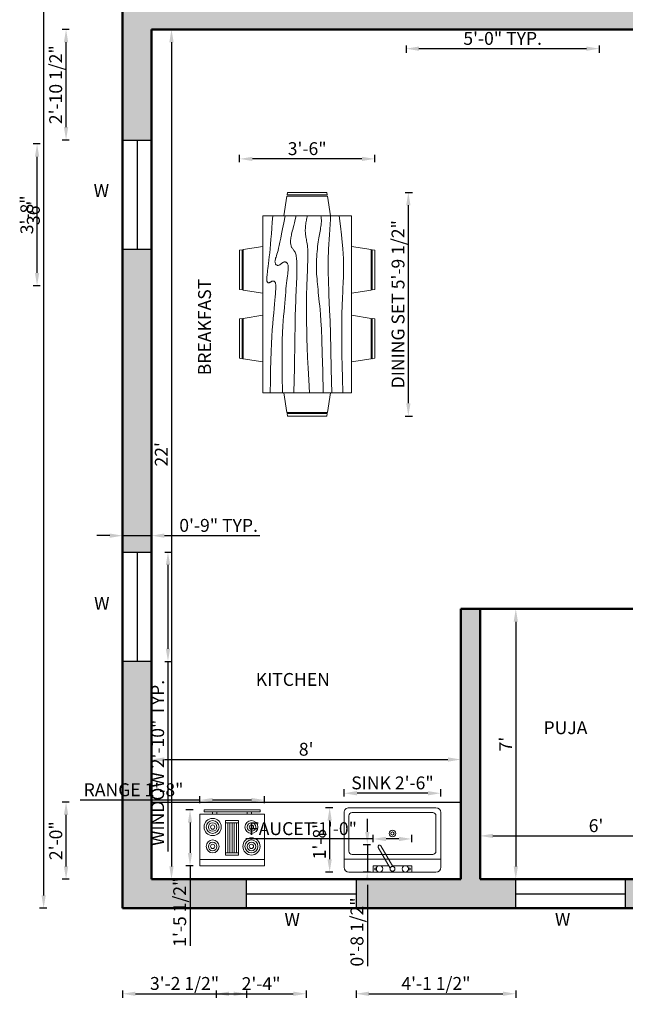
# Model space of a CAD drawing. Units: inches. Extents: x -31 to 511, y -453 to 49.
# Tile 1 of 4: x -31 to 157, y -448 to -142. Entities that reach past the tile are written whole.
import ezdxf

# ---------------------------------------------------------------- set-up
doc = ezdxf.new("R2010")
doc.units = ezdxf.units.IN
for name, color, linetype, lineweight in [('A-ANNO-DIMS', 2, 'Continuous', 18), ('A-ANNO-TEXT', 7, 'Continuous', 18), ('A-AREA-IDEN', 7, 'Continuous', 25), ('A-EQPM', 8, 'Continuous', 18), ('A-FLOR-CASE', 8, 'Continuous', 25), ('A-FLOR-FIXT', 9, 'Continuous', 18), ('A-FURN', 8, 'Continuous', 18), ('A-GLAZ', 4, 'Continuous', 25), ('A-WALL', 7, 'Continuous', 50), ('A-WALL-PATT', 252, 'Continuous', 13)]:
    doc.layers.add(name, color=color, linetype=linetype, lineweight=lineweight)
doc.styles.get("Standard").update_dxf_attribs({"font": 'arial.ttf'})
doc.dimstyles.new('ISO-25', dxfattribs={"dimtxt": 4, "dimasz": 4, "dimexe": 1.25, "dimexo": 0.625, "dimtad": 1, "dimlunit": 3, "dimtxsty": 'Standard', "dimcen": 2.5, "dimadec": 0, "dimazin": 0, "dimtfac": 1, "dimtmove": 0, "dimatfit": 3, "dimfxl": 1, "dimfxlon": 1, "dimarcsym": 0})

# ---------------------------------------------------------------- blocks, each defined once
blk = doc.blocks.new('Sink-single - 30 in top')
blk.add_line((-15, -3.999996), (15, -3.999996))
for points in [[(-13.5, 0), (13.5, 0)], [(-15, -18.499996), (-15, -1.5)], [(15, -1.5), (15, -18.499996)], [(-12.5, -5.499996), (12.5, -5.499996)], [(-13.5, -17.499996), (-13.5, -6.499996)], [(13.5, -6.499996), (13.5, -17.499996)], [(13.5, -19.999996), (-13.5, -19.999996)], [(12.5, -18.499996), (-12.5, -18.499996)]]:
    blk.add_lwpolyline(points)
for radius in [1, 0.5]:
    blk.add_circle((0, -11.999996), radius)
for centre, radius, start, end in [((-13.5, -1.5), 1.5, 90, 180), ((13.5, -1.5), 1.5, 0, 90), ((-12.5, -6.499996), 1, 90, 180), ((12.5, -6.499996), 1, 0, 90), ((-12.5, -17.499996), 1, 180, 270), ((12.5, -17.499996), 1, 270, 0), ((-13.5, -18.499996), 1.5, 180, 270), ((13.5, -18.499996), 1.5, 270, 0)]:
    blk.add_arc(centre, radius, start, end)
blk = doc.blocks.new('Faucet - kit sink top')
for p, q in [((-5.5, -0.75), (-5.5, -1.25)), ((-4.94278, -0.75), (-5.5, -0.75)), ((-5.5, -1.25), (-4.94278, -1.25)), ((-0.14775, -1.7441), (3.56698, -8.1782)), ((4.43301, -7.6782), (0.71828, -1.2441)), ((4.94278, -0.75), (5.5, -0.75)), ((5.5, -1.25), (4.94278, -1.25)), ((5.5, -0.75), (5.5, -1.25))]:
    blk.add_line(p, q)
blk.add_lwpolyline([(-0.00587, -2), (-6, -2), (-6, 0), (6, 0), (6, -2), (1.15195, -2)])
for centre, radius in [((-4, -1), 1), ((4, -1), 1), ((0, -1), 0.75)]:
    blk.add_circle(centre, radius)
blk.add_arc((4, -7.9282), 0.5, 210, 30)
blk = doc.blocks.new('Range-Oven - 30 in top')
for p, q in [((0, -3), (30, -3)), ((12, -6), (18, -6)), ((13, -20), (13, -6)), ((14, -6), (14, -20)), ((15, -20), (15, -6)), ((16, -6), (16, -20)), ((17, -20), (17, -6)), ((18, -20), (12, -20)), ((6, -24), (6, -25)), ((8, -25), (8, -24)), ((22, -25), (22, -24)), ((24, -24), (24, -25))]:
    blk.add_line(p, q)
for points in [[(0, -24), (0, 0), (30, 0), (30, -24)], [(12, -21), (12, -5), (18, -5), (18, -21)], [(2, -26), (2, -25), (28, -25), (28, -26)]]:
    blk.add_lwpolyline(points, close=True)
for centre, radius in [((6, -9), 4), ((6, -9), 3), ((6, -9), 2), ((6, -9), 1), ((24, -9), 3), ((24, -9), 2), ((24, -9), 1), ((6, -18), 3), ((6, -18), 2), ((6, -18), 1), ((24, -18), 4), ((24, -18), 3), ((24, -18), 2), ((24, -18), 1)]:
    blk.add_circle(centre, radius)
blk = doc.blocks.new('Dining Set - 36 x 72 in.')
for p, q in [((-22.2343, 26.00059), (-23.4847, 17.99762)), ((-22.2304, 26), (-5.7608, 26)), ((-22, 27.5), (-22.1562, 26.50042)), ((-5.8416, 26.5), (-22.1534, 26.5)), ((-22, 27.5), (-6, 27.5)), ((-5.8437, 26.49966), (-6, 27.5)), ((-4.5152, 17.99762), (-5.7655, 25.99926)), ((5.7657, 26.00059), (4.5153, 17.99762)), ((5.7696, 26), (22.2392, 26)), ((6, 27.5), (5.8438, 26.50042)), ((22.1584, 26.5), (5.8466, 26.5)), ((6, 27.5), (22, 27.5)), ((22.1563, 26.49966), (22, 27.5)), ((23.4848, 17.99762), (22.2345, 25.99926)), ((36, 18), (-36, 18)), ((-36, 18), (-36, -18)), ((36, -18), (36, 18)), ((-45.5, 8), (-44.5004, 8.15617)), ((-44.5, -8.15843), (-44.5, 8.15338)), ((-44.0006, 8.23428), (-35.9976, 9.48474)), ((-44, 8.23041), (-44, -8.23915)), ((44.0006, 8.23428), (35.9976, 9.48474)), ((44, 8.23041), (44, -8.23915)), ((44.5, -8.15843), (44.5, 8.15338)), ((45.5, 8), (44.5005, 8.15617)), ((-45.5, 8), (-45.5, -8)), ((45.5, 8), (45.5, -8)), ((-44.4997, -8.15631), (-45.5, -8)), ((44.4997, -8.15631), (45.5, -8)), ((-35.9976, -9.48476), (-43.9993, -8.2345)), ((35.9976, -9.48476), (43.9993, -8.2345)), ((-36, -18), (36, -18)), ((-22.2343, -26.0006), (-23.4847, -17.99762)), ((-4.5152, -17.99762), (-5.7655, -25.99928)), ((5.7657, -26.0006), (4.5153, -17.99762)), ((23.4848, -17.99762), (22.2345, -25.99928)), ((-22.2304, -26), (-5.7608, -26)), ((-22, -27.5), (-22.1562, -26.50044)), ((-5.8416, -26.5), (-22.1534, -26.5)), ((-22, -27.5), (-6, -27.5)), ((-5.8437, -26.49967), (-6, -27.5)), ((5.7696, -26), (22.2392, -26)), ((6, -27.5), (5.8438, -26.50044)), ((22.1584, -26.5), (5.8466, -26.5)), ((6, -27.5), (22, -27.5)), ((22.1563, -26.49967), (22, -27.5))]:
    blk.add_line(p, q)
for points in [[(-36, 15), (-31.1772, 14.97754), (-26.8079, 14.91406), (-22.8538, 14.81543), (-19.276, 14.6875), (-16.0362, 14.53613), (-13.0957, 14.36718), (-10.4159, 14.18652), (-7.9583, 14), (-5.6904, 13.81315), (-3.6035, 13.63021), (-1.6954, 13.45508), (0.0365, 13.29166), (1.5945, 13.14388), (2.9811, 13.01562), (4.1988, 12.9108), (5.25, 12.83333), (6.1393, 12.78613), (6.8802, 12.76823), (7.4883, 12.77767), (7.9792, 12.8125), (8.3685, 12.87077), (8.6719, 12.95052), (8.9049, 13.0498), (9.0833, 13.16666), (9.2205, 13.29899), (9.3216, 13.44401), (9.3895, 13.59879), (9.4271, 13.76041), (9.4373, 13.92594), (9.4232, 14.09245), (9.3875, 14.257), (9.3333, 14.41666), (9.2638, 14.56917), (9.1836, 14.71484), (9.0975, 14.85465), (9.0104, 14.98958), (8.9272, 15.1206), (8.8529, 15.2487), (8.7922, 15.37483), (8.75, 15.5), (8.7305, 15.62467), (8.7344, 15.74739), (8.7617, 15.86621), (8.8125, 15.97916), (8.8867, 16.08431), (8.9844, 16.17968), (9.1055, 16.26334), (9.25, 16.33333), (9.4189, 16.38802), (9.6172, 16.42708), (9.8506, 16.45052), (10.125, 16.45833), (10.4463, 16.45052), (10.8203, 16.42708), (11.2529, 16.38802), (11.75, 16.33333), (12.3184, 16.26318), (12.9694, 16.17838), (13.7151, 16.07991), (14.5677, 15.96875), (15.5395, 15.84586), (16.6426, 15.71224), (17.8893, 15.56884), (19.2917, 15.41666), (20.859, 15.25667), (22.5879, 15.08984), (24.4721, 14.91715), (26.5052, 14.73958), (28.6809, 14.5581), (30.9929, 14.3737), (33.4347, 14.18733), (36, 14)], [(-36, 10), (-28.9766, 10.14274), (-23.1725, 10.20442), (-18.4241, 10.19775), (-14.5677, 10.13541), (-11.4399, 10.03011), (-8.877, 9.89453), (-6.7154, 9.74137), (-4.7917, 9.58333), (-2.9698, 9.43082), (-1.2246, 9.28515), (0.4415, 9.14534), (2.026, 9.01041), (3.5266, 8.87939), (4.9408, 8.7513), (6.266, 8.62516), (7.5, 8.5), (8.6411, 8.37549), (9.6914, 8.2539), (10.6538, 8.13818), (11.5312, 8.03125), (12.3267, 7.93603), (13.043, 7.85547), (13.6831, 7.79248), (14.25, 7.75), (14.7471, 7.7303), (15.1797, 7.73307), (15.5537, 7.75732), (15.875, 7.80208), (16.1494, 7.86637), (16.3828, 7.94922), (16.5811, 8.04964), (16.75, 8.16666), (16.8944, 8.29915), (17.0143, 8.44531), (17.1089, 8.60319), (17.1771, 8.77083), (17.218, 8.94629), (17.2305, 9.1276), (17.2137, 9.31282), (17.1667, 9.5), (17.0895, 9.6875), (16.987, 9.875), (16.8649, 10.0625), (16.7292, 10.25), (16.5856, 10.4375), (16.4401, 10.625), (16.2985, 10.8125), (16.1667, 11), (16.05, 11.18733), (15.9518, 11.3737), (15.8752, 11.5581), (15.8229, 11.73958), (15.798, 11.91715), (15.8034, 12.08984), (15.842, 12.25667), (15.9167, 12.41666), (16.0295, 12.56836), (16.1784, 12.70833), (16.3605, 12.83268), (16.5729, 12.9375), (16.8127, 13.01888), (17.0768, 13.07291), (17.3625, 13.0957), (17.6667, 13.08333), (17.9894, 13.03312), (18.3418, 12.94726), (18.7382, 12.82918), (19.1927, 12.68229), (19.7195, 12.51001), (20.3327, 12.31575), (21.0465, 12.10294), (21.875, 11.875), (22.8357, 11.63354), (23.959, 11.37304), (25.2786, 11.08618), (26.8282, 10.76562), (28.6414, 10.40405), (30.752, 9.99414), (33.1936, 9.52856), (36, 9)], [(-36, 5.5), (-30.7157, 5.3348), (-26.069, 5.20963), (-21.9946, 5.11767), (-18.4271, 5.05208), (-15.3009, 5.00602), (-12.5508, 4.97265), (-10.1112, 4.94515), (-7.9167, 4.91666), (-5.909, 4.88167), (-4.0586, 4.83984), (-2.3429, 4.79215), (-0.7396, 4.73958), (0.7739, 4.6831), (2.22, 4.6237), (3.6213, 4.56233), (5, 4.5), (6.373, 4.43782), (7.7344, 4.3776), (9.0723, 4.32129), (10.375, 4.27083), (11.6309, 4.22819), (12.8281, 4.19531), (13.9551, 4.17415), (15, 4.16666), (15.954, 4.17448), (16.819, 4.19791), (17.6001, 4.23698), (18.3021, 4.29166), (18.9299, 4.36198), (19.4883, 4.44791), (19.9823, 4.54948), (20.4167, 4.66666), (20.7969, 4.79899), (21.1302, 4.94401), (21.4245, 5.09879), (21.6875, 5.26041), (21.9271, 5.42594), (22.1511, 5.59245), (22.3672, 5.757), (22.5834, 5.91666), (22.8065, 6.06868), (23.0404, 6.21093), (23.2879, 6.34147), (23.5521, 6.45833), (23.8358, 6.55957), (24.142, 6.64323), (24.4735, 6.70735), (24.8334, 6.75), (25.2235, 6.76969), (25.642, 6.76692), (26.0858, 6.74267), (26.5521, 6.69791), (27.0379, 6.63362), (27.5404, 6.55078), (28.0565, 6.45036), (28.5834, 6.33333), (29.1242, 6.19987), (29.7071, 6.04687), (30.3661, 5.87044), (31.1354, 5.66666), (32.0493, 5.43164), (33.142, 5.16146), (34.4475, 4.85221), (36, 4.5)], [(-36, -1), (-30.7915, -0.6591), (-26.0195, -0.38216), (-21.6519, -0.16284), (-17.6563, 0.00521), (-14.0005, 0.12833), (-10.6523, 0.21289), (-7.5796, 0.26522), (-4.75, 0.29166), (-2.134, 0.29793), (0.2878, 0.28711), (2.5317, 0.26163), (4.6146, 0.22396), (6.5529, 0.17651), (8.3633, 0.12174), (10.0623, 0.06209), (11.6667, 0), (13.1899, -0.06201), (14.6341, -0.1211), (15.9982, -0.17432), (17.2813, -0.21875), (18.4823, -0.25147), (19.6003, -0.26953), (20.6343, -0.27002), (21.5834, -0.25), (22.4481, -0.20768), (23.2357, -0.14584), (23.9549, -0.06836), (24.6146, 0.02083), (25.2235, 0.11784), (25.7904, 0.21875), (26.3241, 0.31966), (26.8334, 0.41666), (27.3265, 0.50618), (27.8099, 0.58593), (28.2894, 0.65397), (28.7709, 0.70833), (29.2601, 0.74707), (29.763, 0.76823), (30.2855, 0.76985), (30.8334, 0.75), (31.4088, 0.70784), (31.9994, 0.64713), (32.589, 0.57275), (33.1615, 0.48958), (33.7008, 0.4025), (34.1908, 0.3164), (34.6153, 0.23616), (34.9584, 0.16666), (35.2099, 0.11165), (35.3848, 0.07031), (35.504, 0.04069), (35.5886, 0.02083), (35.6594, 0.00879), (35.7377, 0.0026), (35.8442, 0.00032), (36, 0)], [(-36, -6.5), (-27.1843, -6.31267), (-20.084, -6.1263), (-14.469, -5.9419), (-10.1094, -5.76042), (-6.7752, -5.58285), (-4.2363, -5.41016), (-2.2629, -5.24333), (-0.625, -5.08334), (0.8708, -4.93099), (2.2715, -4.78646), (3.5872, -4.64974), (4.8281, -4.52084), (6.0046, -4.39974), (7.127, -4.28646), (8.2053, -4.18099), (9.25, -4.08334), (10.2705, -3.99382), (11.2734, -3.91407), (12.2647, -3.84603), (13.25, -3.79167), (14.2354, -3.75293), (15.2266, -3.73177), (16.2295, -3.73015), (17.25, -3.75), (18.2912, -3.79248), (19.3451, -3.85547), (20.4009, -3.93604), (21.4479, -4.03125), (22.4754, -4.13819), (23.4727, -4.25391), (24.4289, -4.37549), (25.3334, -4.5), (26.1785, -4.62492), (26.9694, -4.74935), (27.7145, -4.87281), (28.4219, -4.99479), (29.1, -5.11483), (29.7572, -5.23242), (30.4016, -5.34709), (31.0417, -5.45834), (31.6837, -5.56437), (32.3262, -5.65821), (32.9658, -5.73153), (33.599, -5.77604), (34.2224, -5.78345), (34.8327, -5.74545), (35.4264, -5.65373), (36, -5.5)], [(-36, -10), (-26.4022, -9.81299), (-18.4675, -9.62891), (-11.9839, -9.45069), (-6.7396, -9.28125), (-2.5226, -9.12354), (0.8789, -8.98047), (3.6769, -8.85498), (6.0833, -8.75), (8.2767, -8.66765), (10.3021, -8.60677), (12.1712, -8.56543), (13.8958, -8.54167), (15.4876, -8.53353), (16.9583, -8.53907), (18.3197, -8.55632), (19.5834, -8.58334), (20.7616, -8.61841), (21.8685, -8.66081), (22.9188, -8.71004), (23.9271, -8.76563), (24.9081, -8.82707), (25.8763, -8.89388), (26.8465, -8.96558), (27.8334, -9.04167), (28.8474, -9.12118), (29.8828, -9.20117), (30.93, -9.27824), (31.9792, -9.34896), (33.0205, -9.40991), (34.0443, -9.45768), (35.0407, -9.48885), (36, -9.5)], [(-36, -14.5), (-30.0881, -14.33513), (-25.0332, -14.21224), (-20.7312, -14.12647), (-17.0781, -14.07292), (-13.97, -14.04671), (-11.3027, -14.04297), (-8.9724, -14.05681), (-6.875, -14.08334), (-4.9224, -14.11833), (-3.0905, -14.16016), (-1.3709, -14.20785), (0.2448, -14.26042), (1.7647, -14.3169), (3.1973, -14.3763), (4.5507, -14.43767), (5.8333, -14.5), (7.0554, -14.5621), (8.235, -14.62175), (9.3922, -14.67652), (10.5469, -14.72396), (11.7192, -14.76164), (12.929, -14.78711), (14.1965, -14.79794), (15.5417, -14.79167), (16.9933, -14.76424), (18.6152, -14.70508), (20.4804, -14.60197), (22.6615, -14.44271), (25.2312, -14.21509), (28.2624, -13.9069), (31.8277, -13.50594), (36, -13)]]:
    blk.add_lwpolyline(points)
blk = doc.blocks.new('*D20')
at = {"layer": 'A-ANNO-DIMS', "color": 0, "lineweight": -2, "transparency": 16777216}
for p, q in [((14.65, -145.38), (16.9, -145.38)), ((15.65, -149.38), (15.65, -405.38)), ((14.65, -409.38), (16.9, -409.38))]:
    blk.add_line(p, q, dxfattribs=at)
at = {"layer": 'A-ANNO-DIMS', "color": 0, "transparency": 16777216}
for points in [[(14.98, -149.38), (16.31, -149.38), (15.65, -145.38)], [(14.98, -405.38), (16.31, -405.38), (15.65, -409.38)]]:
    blk.add_solid(points, dxfattribs=at)
at = {"layer": 'Defpoints', "color": 0, "transparency": 16777216}
for p in [(9.46, -145.38), (9.46, -409.38), (15.65, -409.38)]:
    blk.add_point(p, dxfattribs=at)
at = {"layer": 'A-ANNO-DIMS', "color": 0, "transparency": 16777216, "insert": (13.01, -277.38), "char_height": 4, "attachment_point": 5, "rotation": 90}
blk.add_mtext("22'", dxfattribs=at)
blk = doc.blocks.new('*D21')
at = {"layer": 'A-ANNO-DIMS', "color": 0, "lineweight": -2, "transparency": 16777216}
for p, q in [((9.46, -373.17), (9.46, -370.92)), ((13.46, -372.17), (101.46, -372.17)), ((105.46, -373.17), (105.46, -370.92))]:
    blk.add_line(p, q, dxfattribs=at)
at = {"layer": 'A-ANNO-DIMS', "color": 0, "transparency": 16777216}
for points in [[(13.46, -371.5), (13.46, -372.84), (9.46, -372.17)], [(101.46, -371.5), (101.46, -372.84), (105.46, -372.17)]]:
    blk.add_solid(points, dxfattribs=at)
at = {"layer": 'Defpoints', "color": 0, "transparency": 16777216}
for p in [(105.46, -372.17), (9.46, -385.38), (105.46, -385.38)]:
    blk.add_point(p, dxfattribs=at)
at = {"layer": 'A-ANNO-DIMS', "color": 0, "transparency": 16777216, "insert": (57.46, -369.5), "char_height": 4, "attachment_point": 5}
blk.add_mtext("8'", dxfattribs=at)
blk = doc.blocks.new('*D22')
at = {"layer": 'A-ANNO-DIMS', "color": 0, "lineweight": -2, "transparency": 16777216}
for p, q in [((121.55, -325.38), (123.8, -325.38)), ((122.55, -329.38), (122.55, -405.38)), ((121.55, -409.38), (123.8, -409.38))]:
    blk.add_line(p, q, dxfattribs=at)
at = {"layer": 'A-ANNO-DIMS', "color": 0, "transparency": 16777216}
for points in [[(121.89, -329.38), (123.22, -329.38), (122.55, -325.38)], [(121.89, -405.38), (123.22, -405.38), (122.55, -409.38)]]:
    blk.add_solid(points, dxfattribs=at)
at = {"layer": 'Defpoints', "color": 0, "transparency": 16777216}
for p in [(111.46, -325.38), (111.46, -409.38), (122.55, -409.38)]:
    blk.add_point(p, dxfattribs=at)
at = {"layer": 'A-ANNO-DIMS', "color": 0, "transparency": 16777216, "insert": (119.93, -367.38), "char_height": 4, "attachment_point": 5, "rotation": 90}
blk.add_mtext("7'", dxfattribs=at)
blk = doc.blocks.new('*D23')
at = {"layer": 'A-ANNO-DIMS', "color": 0, "lineweight": -2, "transparency": 16777216}
for p, q in [((111.46, -396.89), (111.46, -394.64)), ((115.46, -395.89), (179.46, -395.89)), ((183.46, -396.89), (183.46, -394.64))]:
    blk.add_line(p, q, dxfattribs=at)
at = {"layer": 'A-ANNO-DIMS', "color": 0, "transparency": 16777216}
for points in [[(115.46, -395.23), (115.46, -396.56), (111.46, -395.89)], [(179.46, -395.23), (179.46, -396.56), (183.46, -395.89)]]:
    blk.add_solid(points, dxfattribs=at)
at = {"layer": 'Defpoints', "color": 0, "transparency": 16777216}
for p in [(183.46, -395.89), (111.46, -409.38), (183.46, -409.38)]:
    blk.add_point(p, dxfattribs=at)
at = {"layer": 'A-ANNO-DIMS', "color": 0, "transparency": 16777216, "insert": (147.46, -393.23), "char_height": 4, "attachment_point": 5}
blk.add_mtext("6'", dxfattribs=at)
blk = doc.blocks.new('*D27')
at = {"layer": 'A-ANNO-DIMS', "color": 0, "lineweight": -2, "transparency": 16777216}
for p, q in [((-23.05, 13.62), (-25.3, 13.62)), ((-24.05, 9.62), (-24.05, -414.38)), ((-23.05, -418.38), (-25.3, -418.38))]:
    blk.add_line(p, q, dxfattribs=at)
at = {"layer": 'A-ANNO-DIMS', "color": 0, "transparency": 16777216}
for points in [[(-24.71, 9.62), (-23.38, 9.62), (-24.05, 13.62)], [(-24.71, -414.38), (-23.38, -414.38), (-24.05, -418.38)]]:
    blk.add_solid(points, dxfattribs=at)
at = {"layer": 'Defpoints', "color": 0, "transparency": 16777216}
for p in [(0.46, 13.62), (-24.05, -418.38), (0.46, -418.38)]:
    blk.add_point(p, dxfattribs=at)
at = {"layer": 'A-ANNO-DIMS', "color": 0, "transparency": 16777216, "insert": (-26.72, -202.38), "char_height": 4, "attachment_point": 5, "rotation": 90}
blk.add_mtext("36'", dxfattribs=at)
blk = doc.blocks.new('WIN-34IN')
blk.add_line((0, 4.5), (34, 4.5))
blk.add_lwpolyline([(0, 9), (34, 9), (34, 0), (0, 0)], close=True)
blk = doc.blocks.new('*D30')
at = {"layer": 'A-ANNO-DIMS', "color": 0, "lineweight": -2, "transparency": 16777216}
for p, q in [((13.56, -307.74), (15.81, -307.74)), ((14.56, -311.74), (14.56, -337.74)), ((13.56, -341.74), (15.81, -341.74)), ((14.56, -341.74), (14.56, -400.72))]:
    blk.add_line(p, q, dxfattribs=at)
at = {"layer": 'A-ANNO-DIMS', "color": 0, "transparency": 16777216}
for points in [[(13.9, -311.74), (15.23, -311.74), (14.56, -307.74)], [(13.9, -337.74), (15.23, -337.74), (14.56, -341.74)]]:
    blk.add_solid(points, dxfattribs=at)
at = {"layer": 'Defpoints', "color": 0, "transparency": 16777216}
for p in [(9.46, -307.74), (9.46, -341.74), (14.56, -341.74)]:
    blk.add_point(p, dxfattribs=at)
at = {"layer": 'A-ANNO-DIMS', "color": 0, "transparency": 16777216, "insert": (11.87, -373.23), "char_height": 4, "attachment_point": 5, "rotation": 90}
blk.add_mtext('WINDOW 2\'-10" TYP.', dxfattribs=at)
blk = doc.blocks.new('*D31')
at = {"layer": 'A-ANNO-DIMS', "color": 0, "lineweight": -2, "transparency": 16777216}
for p, q in [((-3.54, -302.64), (-7.54, -302.64)), ((0.46, -303.64), (0.46, -301.39)), ((0.46, -302.64), (9.46, -302.64)), ((9.46, -303.64), (9.46, -301.39)), ((13.46, -302.64), (43.1, -302.64))]:
    blk.add_line(p, q, dxfattribs=at)
at = {"layer": 'A-ANNO-DIMS', "color": 0, "transparency": 16777216}
for points in [[(-3.54, -301.97), (-3.54, -303.31), (0.46, -302.64)], [(13.46, -301.97), (13.46, -303.31), (9.46, -302.64)]]:
    blk.add_solid(points, dxfattribs=at)
at = {"layer": 'Defpoints', "color": 0, "transparency": 16777216}
for p in [(9.46, -302.64), (0.46, -307.74), (9.46, -307.74)]:
    blk.add_point(p, dxfattribs=at)
at = {"layer": 'A-ANNO-DIMS', "color": 0, "transparency": 16777216, "insert": (30.28, -299.97), "char_height": 4, "attachment_point": 5}
blk.add_mtext('0\'-9" TYP.', dxfattribs=at)
blk = doc.blocks.new('*D35')
at = {"layer": 'A-ANNO-DIMS', "color": 0, "lineweight": -2, "transparency": 16777216}
for p, q in [((88.47, -150.38), (88.47, -152.63)), ((144.47, -151.38), (92.47, -151.38)), ((148.47, -150.38), (148.47, -152.63))]:
    blk.add_line(p, q, dxfattribs=at)
at = {"layer": 'A-ANNO-DIMS', "color": 0, "transparency": 16777216}
for points in [[(92.47, -150.71), (92.47, -152.05), (88.47, -151.38)], [(144.47, -150.71), (144.47, -152.05), (148.47, -151.38)]]:
    blk.add_solid(points, dxfattribs=at)
at = {"layer": 'Defpoints', "color": 0, "transparency": 16777216}
for p in [(88.47, -139.38), (148.47, -139.38), (88.47, -151.38)]:
    blk.add_point(p, dxfattribs=at)
at = {"layer": 'A-ANNO-DIMS', "color": 0, "transparency": 16777216, "insert": (118.47, -148.71), "char_height": 4, "attachment_point": 5}
blk.add_mtext('5\'-0" TYP.', dxfattribs=at)
blk = doc.blocks.new('*D40')
at = {"layer": 'A-ANNO-DIMS', "color": 0, "lineweight": -2, "transparency": 16777216}
for p, q in [((88.19, -196.03), (90.44, -196.03)), ((89.19, -261.49), (89.19, -200.03)), ((88.19, -265.49), (90.44, -265.49))]:
    blk.add_line(p, q, dxfattribs=at)
at = {"layer": 'A-ANNO-DIMS', "color": 0, "transparency": 16777216}
for points in [[(88.52, -200.03), (89.86, -200.03), (89.19, -196.03)], [(88.52, -261.49), (89.86, -261.49), (89.19, -265.49)]]:
    blk.add_solid(points, dxfattribs=at)
at = {"layer": 'Defpoints', "color": 0, "transparency": 16777216}
for p in [(78.77, -196.03), (89.19, -196.03), (78.77, -265.49)]:
    blk.add_point(p, dxfattribs=at)
at = {"layer": 'A-ANNO-DIMS', "color": 0, "transparency": 16777216, "insert": (86.5, -230.76), "char_height": 4, "attachment_point": 5, "rotation": 90}
blk.add_mtext('DINING SET 5\'-9 1/2"', dxfattribs=at)
blk = doc.blocks.new('*D41')
at = {"layer": 'A-ANNO-DIMS', "color": 0, "lineweight": -2, "transparency": 16777216}
for p, q in [((36.79, -186.61), (36.79, -184.36)), ((74.77, -185.61), (40.79, -185.61)), ((78.77, -186.61), (78.77, -184.36))]:
    blk.add_line(p, q, dxfattribs=at)
at = {"layer": 'A-ANNO-DIMS', "color": 0, "transparency": 16777216}
for points in [[(40.79, -184.95), (40.79, -186.28), (36.79, -185.61)], [(74.77, -184.95), (74.77, -186.28), (78.77, -185.61)]]:
    blk.add_solid(points, dxfattribs=at)
at = {"layer": 'Defpoints', "color": 0, "transparency": 16777216}
for p in [(36.79, -185.61), (36.79, -196.03), (78.77, -196.03)]:
    blk.add_point(p, dxfattribs=at)
at = {"layer": 'A-ANNO-DIMS', "color": 0, "transparency": 16777216, "insert": (57.78, -182.95), "char_height": 4, "attachment_point": 5}
blk.add_mtext('3\'-6"', dxfattribs=at)
blk = doc.blocks.new('*D42')
at = {"layer": 'A-ANNO-DIMS', "color": 0, "lineweight": -2, "transparency": 16777216}
for p, q in [((24.42, -384.77), (-12.68, -384.77)), ((24.42, -385.77), (24.42, -383.52)), ((40.49, -384.77), (28.42, -384.77)), ((44.49, -385.77), (44.49, -383.52))]:
    blk.add_line(p, q, dxfattribs=at)
at = {"layer": 'A-ANNO-DIMS', "color": 0, "transparency": 16777216}
for points in [[(28.42, -384.1), (28.42, -385.44), (24.42, -384.77)], [(40.49, -384.1), (40.49, -385.44), (44.49, -384.77)]]:
    blk.add_solid(points, dxfattribs=at)
at = {"layer": 'Defpoints', "color": 0, "transparency": 16777216}
for p in [(24.42, -384.77), (24.42, -387.78), (44.49, -387.78)]:
    blk.add_point(p, dxfattribs=at)
at = {"layer": 'A-ANNO-DIMS', "color": 0, "transparency": 16777216, "insert": (3.87, -382.08), "char_height": 4, "attachment_point": 5}
blk.add_mtext('RANGE 1\'-8"', dxfattribs=at)
blk = doc.blocks.new('*D43')
at = {"layer": 'A-ANNO-DIMS', "color": 0, "lineweight": -2, "transparency": 16777216}
for p, q in [((22.4, -387.78), (20.15, -387.78)), ((21.4, -391.78), (21.4, -401.18)), ((22.4, -405.18), (20.15, -405.18)), ((21.4, -405.18), (21.4, -430.01))]:
    blk.add_line(p, q, dxfattribs=at)
at = {"layer": 'A-ANNO-DIMS', "color": 0, "transparency": 16777216}
for points in [[(20.74, -391.78), (22.07, -391.78), (21.4, -387.78)], [(20.74, -401.18), (22.07, -401.18), (21.4, -405.18)]]:
    blk.add_solid(points, dxfattribs=at)
at = {"layer": 'Defpoints', "color": 0, "transparency": 16777216}
for p in [(24.42, -387.78), (21.4, -405.18), (24.42, -405.18)]:
    blk.add_point(p, dxfattribs=at)
at = {"layer": 'A-ANNO-DIMS', "color": 0, "transparency": 16777216, "insert": (18.71, -419.59), "char_height": 4, "attachment_point": 5, "rotation": 90}
blk.add_mtext('1\'-5 1/2"', dxfattribs=at)
blk = doc.blocks.new('*D44')
at = {"layer": 'A-ANNO-DIMS', "color": 0, "lineweight": -2, "transparency": 16777216}
for p, q in [((69.26, -383.64), (69.26, -381.39)), ((99.26, -383.64), (99.26, -381.39)), ((95.26, -382.64), (73.26, -382.64))]:
    blk.add_line(p, q, dxfattribs=at)
at = {"layer": 'A-ANNO-DIMS', "color": 0, "transparency": 16777216}
for points in [[(73.26, -381.97), (73.26, -383.31), (69.26, -382.64)], [(95.26, -381.97), (95.26, -383.31), (99.26, -382.64)]]:
    blk.add_solid(points, dxfattribs=at)
at = {"layer": 'Defpoints', "color": 0, "transparency": 16777216}
for p in [(69.26, -382.64), (69.26, -387.14), (99.26, -387.14)]:
    blk.add_point(p, dxfattribs=at)
at = {"layer": 'A-ANNO-DIMS', "color": 0, "transparency": 16777216, "insert": (84.26, -379.95), "char_height": 4, "attachment_point": 5}
blk.add_mtext('SINK 2\'-6"', dxfattribs=at)
blk = doc.blocks.new('*D45')
at = {"layer": 'A-ANNO-DIMS', "color": 0, "lineweight": -2, "transparency": 16777216}
for p, q in [((65.76, -387.14), (63.51, -387.14)), ((64.76, -391.14), (64.76, -403.14)), ((65.76, -407.14), (63.51, -407.14))]:
    blk.add_line(p, q, dxfattribs=at)
at = {"layer": 'A-ANNO-DIMS', "color": 0, "transparency": 16777216}
for points in [[(64.09, -391.14), (65.42, -391.14), (64.76, -387.14)], [(64.09, -403.14), (65.42, -403.14), (64.76, -407.14)]]:
    blk.add_solid(points, dxfattribs=at)
at = {"layer": 'Defpoints', "color": 0, "transparency": 16777216}
for p in [(69.26, -387.14), (64.76, -407.14), (69.26, -407.14)]:
    blk.add_point(p, dxfattribs=at)
at = {"layer": 'A-ANNO-DIMS', "color": 0, "transparency": 16777216, "insert": (62.09, -397.14), "char_height": 4, "attachment_point": 5, "rotation": 90}
blk.add_mtext('1\'-8"', dxfattribs=at)
blk = doc.blocks.new('*D46')
at = {"layer": 'A-ANNO-DIMS', "color": 0, "lineweight": -2, "transparency": 16777216}
for p, q in [((78.26, -396.84), (38.7, -396.84)), ((78.26, -397.84), (78.26, -395.59)), ((86.26, -396.84), (82.26, -396.84)), ((90.26, -397.84), (90.26, -395.59))]:
    blk.add_line(p, q, dxfattribs=at)
at = {"layer": 'A-ANNO-DIMS', "color": 0, "transparency": 16777216}
for points in [[(82.26, -396.17), (82.26, -397.51), (78.26, -396.84)], [(86.26, -396.17), (86.26, -397.51), (90.26, -396.84)]]:
    blk.add_solid(points, dxfattribs=at)
at = {"layer": 'Defpoints', "color": 0, "transparency": 16777216}
for p in [(78.26, -396.84), (78.26, -398.64), (90.26, -398.64)]:
    blk.add_point(p, dxfattribs=at)
at = {"layer": 'A-ANNO-DIMS', "color": 0, "transparency": 16777216, "insert": (56.48, -394.15), "char_height": 4, "attachment_point": 5}
blk.add_mtext('FAUCET 1\'-0"', dxfattribs=at)
blk = doc.blocks.new('*D47')
at = {"layer": 'A-ANNO-DIMS', "color": 0, "lineweight": -2, "transparency": 16777216}
for p, q in [((76.46, -394.64), (76.46, -390.64)), ((77.46, -398.64), (75.21, -398.64)), ((76.46, -398.64), (76.46, -407.14)), ((77.46, -407.14), (75.21, -407.14)), ((76.46, -411.14), (76.46, -436.34))]:
    blk.add_line(p, q, dxfattribs=at)
at = {"layer": 'A-ANNO-DIMS', "color": 0, "transparency": 16777216}
for points in [[(75.79, -394.64), (77.12, -394.64), (76.46, -398.64)], [(75.79, -411.14), (77.12, -411.14), (76.46, -407.14)]]:
    blk.add_solid(points, dxfattribs=at)
at = {"layer": 'Defpoints', "color": 0, "transparency": 16777216}
for p in [(78.26, -398.64), (76.46, -407.14), (78.26, -407.14)]:
    blk.add_point(p, dxfattribs=at)
at = {"layer": 'A-ANNO-DIMS', "color": 0, "transparency": 16777216, "insert": (73.76, -425.74), "char_height": 4, "attachment_point": 5, "rotation": 90}
blk.add_mtext('0\'-8 1/2"', dxfattribs=at)
blk = doc.blocks.new('*D57')
at = {"layer": 'A-ANNO-DIMS', "color": 0, "lineweight": -2, "transparency": 16777216}
for p, q in [((-16.09, -145.38), (-18.34, -145.38)), ((-17.09, -175.76), (-17.09, -149.38)), ((-16.09, -179.76), (-18.34, -179.76))]:
    blk.add_line(p, q, dxfattribs=at)
at = {"layer": 'A-ANNO-DIMS', "color": 0, "transparency": 16777216}
for points in [[(-17.75, -149.38), (-16.42, -149.38), (-17.09, -145.38)], [(-17.75, -175.76), (-16.42, -175.76), (-17.09, -179.76)]]:
    blk.add_solid(points, dxfattribs=at)
at = {"layer": 'Defpoints', "color": 0, "transparency": 16777216}
for p in [(-17.09, -145.38), (9.46, -145.38), (9.46, -179.76)]:
    blk.add_point(p, dxfattribs=at)
at = {"layer": 'A-ANNO-DIMS', "color": 0, "transparency": 16777216, "insert": (-19.78, -162.57), "char_height": 4, "attachment_point": 5, "rotation": 90}
blk.add_mtext('2\'-10 1/2"', dxfattribs=at)
blk = doc.blocks.new('*D58')
at = {"layer": 'A-ANNO-DIMS', "color": 0, "lineweight": -2, "transparency": 16777216}
for p, q in [((508.55, -213.76), (510.8, -213.76)), ((509.55, -217.76), (509.55, -303.74)), ((508.55, -307.74), (510.8, -307.74))]:
    blk.add_line(p, q, dxfattribs=at)
at = {"layer": 'A-ANNO-DIMS', "color": 0, "transparency": 16777216}
for points in [[(508.88, -217.76), (510.22, -217.76), (509.55, -213.76)], [(508.88, -303.74), (510.22, -303.74), (509.55, -307.74)]]:
    blk.add_solid(points, dxfattribs=at)
at = {"layer": 'Defpoints', "color": 0, "transparency": 16777216}
for p in [(9.46, -213.76), (9.46, -307.74), (509.55, -307.74)]:
    blk.add_point(p, dxfattribs=at)
at = {"layer": 'A-ANNO-DIMS', "color": 0, "transparency": 16777216, "insert": (506.88, -260.75), "char_height": 4, "attachment_point": 5, "rotation": 90}
blk.add_mtext('7\'-10"', dxfattribs=at)
blk = doc.blocks.new('*D59')
at = {"layer": 'A-ANNO-DIMS', "color": 0, "lineweight": -2, "transparency": 16777216}
for p, q in [((0.46, -443.93), (0.46, -446.18)), ((4.46, -444.93), (34.94, -444.93)), ((38.94, -443.93), (38.94, -446.18))]:
    blk.add_line(p, q, dxfattribs=at)
at = {"layer": 'A-ANNO-DIMS', "color": 0, "transparency": 16777216}
for points in [[(4.46, -444.26), (4.46, -445.6), (0.46, -444.93)], [(34.94, -444.26), (34.94, -445.6), (38.94, -444.93)]]:
    blk.add_solid(points, dxfattribs=at)
at = {"layer": 'Defpoints', "color": 0, "transparency": 16777216}
for p in [(0.46, -418.38), (38.94, -418.38), (38.94, -444.93)]:
    blk.add_point(p, dxfattribs=at)
at = {"layer": 'A-ANNO-DIMS', "color": 0, "transparency": 16777216, "insert": (19.7, -442.24), "char_height": 4, "attachment_point": 5}
blk.add_mtext('3\'-2 1/2"', dxfattribs=at)
blk = doc.blocks.new('*D60')
at = {"layer": 'A-ANNO-DIMS', "color": 0, "lineweight": -2, "transparency": 16777216}
for p, q in [((72.94, -443.93), (72.94, -446.18)), ((76.94, -444.93), (118.55, -444.93)), ((122.55, -443.93), (122.55, -446.18))]:
    blk.add_line(p, q, dxfattribs=at)
at = {"layer": 'A-ANNO-DIMS', "color": 0, "transparency": 16777216}
for points in [[(76.94, -444.26), (76.94, -445.6), (72.94, -444.93)], [(118.55, -444.26), (118.55, -445.6), (122.55, -444.93)]]:
    blk.add_solid(points, dxfattribs=at)
at = {"layer": 'Defpoints', "color": 0, "transparency": 16777216}
for p in [(72.94, -418.38), (122.55, -418.38), (122.55, -444.93)]:
    blk.add_point(p, dxfattribs=at)
at = {"layer": 'A-ANNO-DIMS', "color": 0, "transparency": 16777216, "insert": (97.75, -442.24), "char_height": 4, "attachment_point": 5}
blk.add_mtext('4\'-1 1/2"', dxfattribs=at)
blk = doc.blocks.new('*D64')
at = {"layer": 'A-ANNO-DIMS', "color": 0, "lineweight": -2, "transparency": 16777216}
for p, q in [((-16.09, -385.38), (-18.34, -385.38)), ((-17.09, -405.38), (-17.09, -389.38)), ((-16.09, -409.38), (-18.34, -409.38))]:
    blk.add_line(p, q, dxfattribs=at)
at = {"layer": 'A-ANNO-DIMS', "color": 0, "transparency": 16777216}
for points in [[(-17.75, -389.38), (-16.42, -389.38), (-17.09, -385.38)], [(-17.75, -405.38), (-16.42, -405.38), (-17.09, -409.38)]]:
    blk.add_solid(points, dxfattribs=at)
at = {"layer": 'Defpoints', "color": 0, "transparency": 16777216}
for p in [(-17.09, -385.38), (9.46, -385.38), (9.46, -409.38)]:
    blk.add_point(p, dxfattribs=at)
at = {"layer": 'A-ANNO-DIMS', "color": 0, "transparency": 16777216, "insert": (-19.75, -397.38), "char_height": 4, "attachment_point": 5, "rotation": 90}
blk.add_mtext('2\'-0"', dxfattribs=at)
blk = doc.blocks.new('*D65')
at = {"layer": 'A-ANNO-DIMS', "color": 0, "lineweight": -2, "transparency": 16777216}
for p, q in [((29.47, -443.93), (29.47, -446.18)), ((33.47, -444.93), (53.47, -444.93)), ((57.47, -443.93), (57.47, -446.18))]:
    blk.add_line(p, q, dxfattribs=at)
at = {"layer": 'A-ANNO-DIMS', "color": 0, "transparency": 16777216}
for points in [[(33.47, -444.26), (33.47, -445.6), (29.47, -444.93)], [(53.47, -444.26), (53.47, -445.6), (57.47, -444.93)]]:
    blk.add_solid(points, dxfattribs=at)
at = {"layer": 'Defpoints', "color": 0, "transparency": 16777216}
for p in [(29.47, -67.58), (57.47, -78.08), (57.47, -444.93)]:
    blk.add_point(p, dxfattribs=at)
at = {"layer": 'A-ANNO-DIMS', "color": 0, "transparency": 16777216, "insert": (43.47, -442.3), "char_height": 4, "attachment_point": 5}
blk.add_mtext('2\'-4"', dxfattribs=at)
blk = doc.blocks.new('*D68')
at = {"layer": 'A-ANNO-DIMS', "color": 0, "lineweight": -2, "transparency": 16777216}
for p, q in [((-25.09, -180.94), (-27.34, -180.94)), ((-26.09, -221.03), (-26.09, -184.94)), ((-25.09, -225.03), (-27.34, -225.03))]:
    blk.add_line(p, q, dxfattribs=at)
at = {"layer": 'A-ANNO-DIMS', "color": 0, "transparency": 16777216}
for points in [[(-26.75, -184.94), (-25.42, -184.94), (-26.09, -180.94)], [(-26.75, -221.03), (-25.42, -221.03), (-26.09, -225.03)]]:
    blk.add_solid(points, dxfattribs=at)
at = {"layer": 'Defpoints', "color": 0, "transparency": 16777216}
for p in [(-26.09, -180.94), (299.69, -180.94), (299.69, -225.03)]:
    blk.add_point(p, dxfattribs=at)
at = {"layer": 'A-ANNO-DIMS', "color": 0, "transparency": 16777216, "insert": (-28.75, -202.99), "char_height": 4, "attachment_point": 5, "rotation": 90}
blk.add_mtext('3\'-8"', dxfattribs=at)

msp = doc.modelspace()

# ---------------------------------------------------------------- hatches: boundary and pattern name
at = {"layer": 'A-WALL-PATT'}
h = msp.add_hatch(color=256, dxfattribs=at)
h.dxf.hatch_style = 1
h.paths.add_polyline_path([(122.408, 13.62), (0.465, 13.62), (0.465, -55.742), (9.465, -55.742), (9.465, 4.62), (57.465, 4.62), (57.465, 0.62), (59.528, 0.62), (63.465, 0.62), (63.465, 4.62), (122.408, 4.62)])
h.paths.add_polyline_path([(267.569, 13.62), (156.408, 13.62), (156.408, 4.62), (207.465, 4.62), (207.465, -139.38), (203.465, -139.38), (203.465, -140.534), (203.465, -145.38), (217.465, -145.38), (217.465, -140.567), (217.465, -139.38), (213.465, -139.38), (213.465, 4.62), (267.569, 4.62)])
h.paths.add_polyline_path([(432.465, 13.62), (301.569, 13.62), (301.569, 4.62), (357.465, 4.62), (357.465, 0.312), (361.402, 0.312), (363.465, 0.312), (363.465, 4.62), (423.465, 4.62), (423.465, -55.742), (432.465, -55.742)])
h.paths.add_polyline_path([(432.465, -73.742), (423.465, -73.742), (423.465, -139.38), (363.465, -139.38), (363.465, -29.688), (357.465, -29.688), (357.465, -139.38), (253.542, -139.38, -0.0082235), (253.561, -140.567), (253.561, -145.38), (423.465, -145.38), (423.465, -409.38), (414.601, -409.38), (414.601, -412.759), (414.601, -418.38), (432.465, -418.38)])
h.paths.add_polyline_path([(167.12, -140.534, -0.00794), (167.139, -139.38), (63.465, -139.38), (63.465, -29.38), (57.465, -29.38), (57.465, -57.083), (57.472, -57.083), (57.472, -78.083), (57.465, -139.38), (9.465, -139.38), (9.465, -73.742), (0.465, -73.742), (0.465, -179.759), (9.465, -179.759), (9.465, -145.38), (167.12, -145.38)])
h.paths.add_polyline_path([(372.446, -412.759, -0.0200643), (372.581, -409.38), (327.465, -409.38), (327.465, -265.38), (285.454, -265.38), (285.454, -271.38), (321.465, -271.38), (321.465, -409.38), (273.096, -409.38), (273.096, -418.38), (372.446, -418.38)], flags=17)
h.paths.add_polyline_path([(239.096, -409.38), (189.465, -409.38), (189.465, -271.38), (243.454, -271.38), (243.454, -265.38), (183.465, -265.38), (183.465, -409.38), (156.552, -409.38), (156.552, -418.38), (239.096, -418.38)])
h.paths.add_polyline_path([(122.552, -409.38), (111.465, -409.38), (111.465, -325.38), (105.465, -325.38), (105.465, -409.38), (72.938, -409.38), (72.938, -418.38), (122.552, -418.38)])
h.paths.add_polyline_path([(38.938, -409.38), (9.465, -409.38), (9.465, -341.741), (0.465, -341.741), (0.465, -418.38), (38.938, -418.38)])
h.paths.add_polyline_path([(9.465, -213.759), (0.465, -213.759), (0.465, -307.741), (9.465, -307.741)])

# ---------------------------------------------------------------- linework, layer by layer
at = {"layer": 'A-FLOR-CASE'}
msp.add_line((9.465, -385.38), (105.465, -385.38), dxfattribs=at)
at = {"layer": 'A-WALL'}
for p, q in [((0.465, -418.38), (0.465, 13.62)), ((9.465, -409.38), (9.465, -145.38)), ((9.465, -145.38), (423.465, -145.38)), ((105.465, -409.38), (105.465, -325.38)), ((105.465, -325.38), (111.465, -325.38)), ((105.465, -325.38), (183.465, -325.38)), ((111.465, -325.38), (111.465, -409.38)), ((105.465, -409.38), (9.465, -409.38)), ((183.465, -409.38), (111.465, -409.38)), ((432.465, -418.38), (0.465, -418.38))]:
    msp.add_line(p, q, dxfattribs=at)

# ---------------------------------------------------------------- block references
at = {"layer": 'A-EQPM', "xscale": 0.6691867825349315, "yscale": 0.6691867825349315, "zscale": 0.6691867825349315, "rotation": 180}
msp.add_blockref('Range-Oven - 30 in top', (44.491, -405.18), dxfattribs=at)
at = {"layer": 'A-FLOR-FIXT', "rotation": 180}
for name in ['Sink-single - 30 in top', 'Faucet - kit sink top']:
    msp.add_blockref(name, (84.257, -407.14), dxfattribs=at)
at = {"layer": 'A-FURN', "xscale": 0.7632333908399709, "yscale": 0.7632333908399709, "zscale": 0.7632333908399709, "rotation": 90}
msp.add_blockref('Dining Set - 36 x 72 in.', (57.783, -230.759), dxfattribs=at)
at = {"layer": 'A-GLAZ'}
for p, rotation in [((0.465, -179.76), 270), ((0.465, -307.741), 270.0000000000001)]:
    msp.add_blockref('WIN-34IN', p, dxfattribs=dict(at, rotation=rotation))
for p in [(38.939, -418.38), (122.552, -418.38)]:
    msp.add_blockref('WIN-34IN', p, dxfattribs=at)

# ---------------------------------------------------------------- texts
at = {"layer": 'A-ANNO-TEXT', "char_height": 4, "attachment_point": 1}
for width, insert in [(5.86547, (-8.521, -193.463)), (5.4606, (-8.371, -321.671)), (9.21101, (50.734, -419.846)), (12.0965, (134.708, -419.797))]:
    msp.add_mtext_dynamic_manual_height_columns('W', width=width, gutter_width=12.5, heights=[0], dxfattribs=dict(at, insert=insert))
at = {"layer": 'A-AREA-IDEN', "insert": (23.917, -252.81), "char_height": 4, "attachment_point": 1, "rotation": 90}
msp.add_mtext_dynamic_manual_height_columns('BREAKFAST', width=68.72849, gutter_width=12.5, heights=[0], dxfattribs=at)
at = {"layer": 'A-AREA-IDEN', "char_height": 4, "attachment_point": 1}
for s, width, insert in [('KITCHEN', 53.4476, (41.815, -345.3)), ('PUJA', 38.29594, (131.163, -360.289))]:
    msp.add_mtext_dynamic_manual_height_columns(s, width=width, gutter_width=12.5, heights=[0], dxfattribs=dict(at, insert=insert))

# ---------------------------------------------------------------- dimensions: what is measured, and where the dimension line sits
at = {"layer": 'A-ANNO-DIMS'}
for base, p1, p2, angle, override, picture, middle in [((-24.047, -418.38), (0.465, 13.62), (0.465, -418.38), 90, {"dimclrd": 0, "dimclre": 0, "dimclrt": 0}, '*D27', (-26.716, -202.38)), ((-17.085, -145.38), (9.465, -179.759), (9.465, -145.38), 90, {"dimdec": 1, "dimlfac": 1, "dimrnd": 0, "dimzin": 1, "dimdsep": 46, "dimlunit": 4, "dimfrac": 2}, '*D57', (-19.778, -162.569)), ((15.647, -409.38), (9.465, -145.38), (9.465, -409.38), 90, {"dimclrd": 0, "dimclre": 0, "dimclrt": 0}, '*D20', (13.014, -277.38)), ((36.794, -185.614), (78.771, -196.032), (36.794, -196.032), 180, {"dimdec": 1, "dimlfac": 1, "dimrnd": 0, "dimzin": 1, "dimdsep": 46, "dimlunit": 4, "dimfrac": 2}, '*D41', (57.783, -182.945)), ((-26.085, -180.941), (299.695, -225.033), (299.695, -180.941), 90, {"dimdec": 1, "dimlfac": 1, "dimrnd": 0, "dimzin": 1, "dimdsep": 46, "dimlunit": 4, "dimfrac": 2}, '*D68', (-28.754, -202.987)), ((509.551, -307.741), (9.465, -213.759), (9.465, -307.741), 90, {"dimdec": 1, "dimlfac": 1, "dimrnd": 0, "dimzin": 1, "dimdsep": 46, "dimlunit": 4, "dimfrac": 2}, '*D58', (506.883, -260.75)), ((122.552, -409.38), (111.465, -325.38), (111.465, -409.38), 90, {"dimclrd": 0, "dimclre": 0, "dimclrt": 0}, '*D22', (119.927, -367.38)), ((-17.085, -385.38), (9.465, -409.38), (9.465, -385.38), 90, {"dimdec": 1, "dimlfac": 1, "dimrnd": 0, "dimzin": 1, "dimdsep": 46, "dimlunit": 4, "dimfrac": 2}, '*D64', (-19.753, -397.38)), ((21.404, -405.18), (24.415, -387.781), (24.415, -405.18), 270, {"dimdec": 1, "dimlfac": 1, "dimrnd": 0, "dimzin": 1, "dimdsep": 46, "dimlunit": 4, "dimfrac": 2}, '*D43', (18.711, -419.594)), ((64.757, -407.14), (69.257, -387.14), (69.257, -407.14), 270, {"dimdec": 1, "dimlfac": 1, "dimrnd": 0, "dimzin": 1, "dimdsep": 46, "dimlunit": 4, "dimfrac": 2}, '*D45', (62.089, -397.14)), ((76.457, -407.14), (78.257, -398.641), (78.257, -407.14), 270, {"dimdec": 1, "dimlfac": 1, "dimrnd": 0, "dimzin": 1, "dimdsep": 46, "dimlunit": 4, "dimfrac": 2}, '*D47', (73.763, -425.742))]:
    dim = msp.add_linear_dim(base=base, p1=p1, p2=p2, angle=angle, dimstyle='ISO-25', override=override, dxfattribs=at)
    dim.commit()
    dim.dimension.update_dxf_attribs({"geometry": picture, "text_midpoint": middle})
for base, p1, p2, override, picture, middle in [((57.472, -444.93), (29.472, -67.583), (57.472, -78.083), {"dimdec": 1, "dimlfac": 1, "dimrnd": 0, "dimzin": 1, "dimdsep": 46, "dimlunit": 4, "dimfrac": 2}, '*D65', (43.472, -442.297)), ((105.465, -372.169), (9.465, -385.38), (105.465, -385.38), {"dimclrd": 0, "dimclre": 0, "dimclrt": 0}, '*D21', (57.465, -369.501)), ((183.465, -395.893), (111.465, -409.38), (183.465, -409.38), {"dimclrd": 0, "dimclre": 0, "dimclrt": 0}, '*D23', (147.465, -393.226)), ((38.938, -444.93), (0.465, -418.38), (38.938, -418.38), {"dimdec": 1, "dimlfac": 1, "dimrnd": 0, "dimzin": 1, "dimdsep": 46, "dimlunit": 4, "dimfrac": 2}, '*D59', (19.702, -442.235)), ((122.552, -444.93), (72.938, -418.38), (122.552, -418.38), {"dimdec": 1, "dimlfac": 1, "dimrnd": 0, "dimzin": 1, "dimdsep": 46, "dimlunit": 4, "dimfrac": 2}, '*D60', (97.745, -442.237))]:
    dim = msp.add_linear_dim(base=base, p1=p1, p2=p2, dimstyle='ISO-25', override=override, dxfattribs=at)
    dim.commit()
    dim.dimension.update_dxf_attribs({"geometry": picture, "text_midpoint": middle})
for base, p1, p2, angle, text, picture, middle in [((88.466, -151.38), (148.466, -139.38), (88.466, -139.38), 180, '<> TYP.', '*D35', (118.466, -148.712)), ((89.19, -196.032), (78.771, -265.486), (78.771, -196.032), 90, 'DINING SET <>', '*D40', (86.496, -230.759)), ((14.565, -341.741), (9.465, -307.741), (9.465, -341.741), 270, 'WINDOW <> TYP.', '*D30', (11.87, -373.228)), ((24.415, -384.77), (44.491, -387.781), (24.415, -387.781), 180, 'RANGE <>', '*D42', (3.865, -382.077)), ((69.257, -382.64), (99.257, -387.14), (69.257, -387.14), 180, 'SINK <>', '*D44', (84.257, -379.947)), ((78.257, -396.841), (90.257, -398.641), (78.257, -398.641), 180, 'FAUCET <>', '*D46', (56.476, -394.148))]:
    dim = msp.add_linear_dim(base=base, p1=p1, p2=p2, angle=angle, text=text, dimstyle='ISO-25', override={"dimdec": 1, "dimlfac": 1, "dimrnd": 0, "dimzin": 1, "dimdsep": 46, "dimlunit": 4, "dimfrac": 2}, dxfattribs=at)
    dim.commit()
    dim.dimension.update_dxf_attribs({"geometry": picture, "text_midpoint": middle})
dim = msp.add_linear_dim(base=(9.465, -302.641), p1=(0.465, -307.741), p2=(9.465, -307.741), text='<> TYP.', dimstyle='ISO-25', override={"dimdec": 1, "dimlfac": 1, "dimrnd": 0, "dimzin": 1, "dimdsep": 46, "dimlunit": 4, "dimfrac": 2}, dxfattribs=at)
dim.commit()
dim.dimension.update_dxf_attribs({"geometry": '*D31', "text_midpoint": (30.281, -299.974)})

doc.saveas('drawing.dxf')
